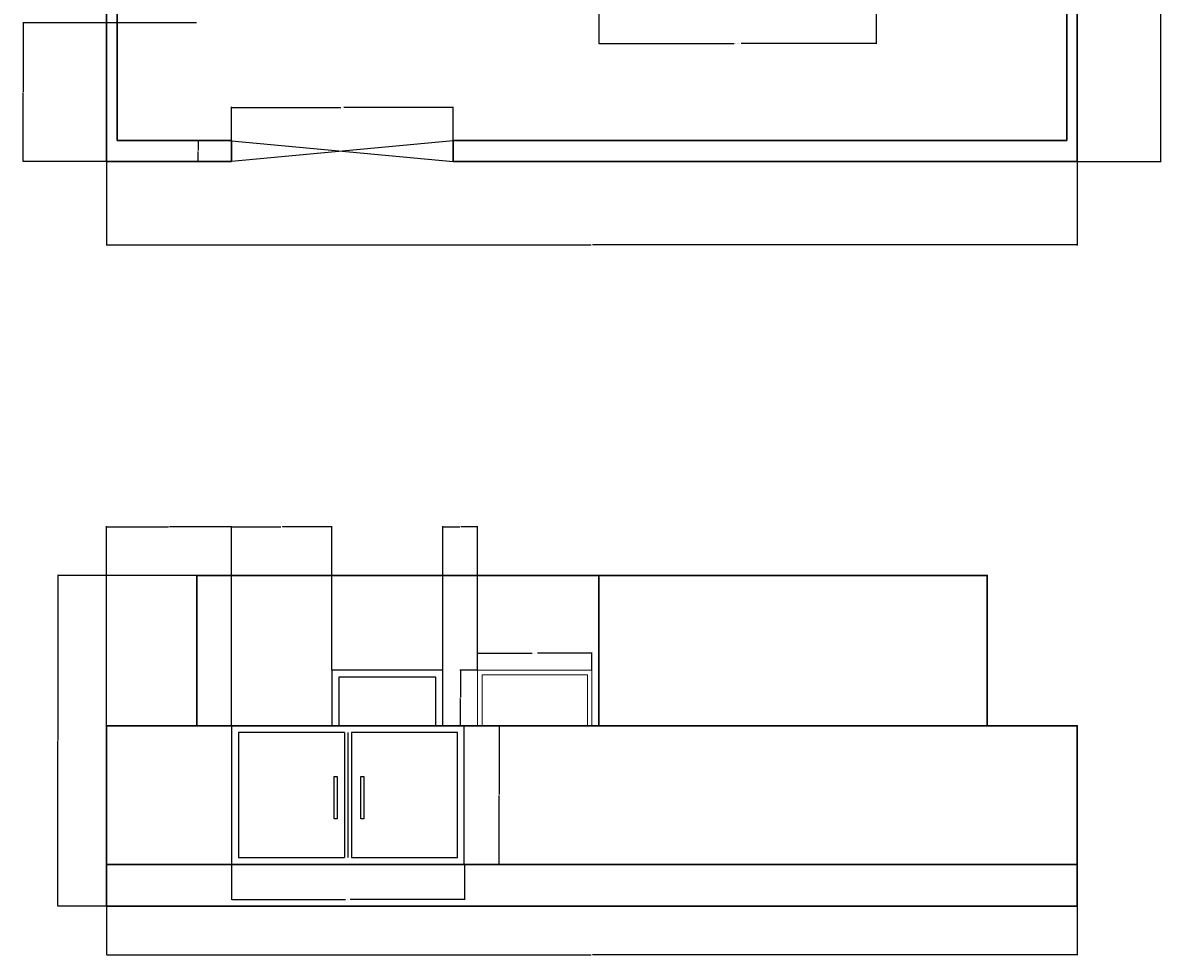
# Model space of a CAD drawing. Units: inches. Extents: x 810 to 2232, y 728 to 1827.
# Tile 1 of 6: x 810 to 1302, y 728 to 1131. Entities that reach past the tile are written whole.
import ezdxf

# ---------------------------------------------------------------- set-up
doc = ezdxf.new("R2010")
doc.units = ezdxf.units.IN
for name, color, linetype, lineweight in [('A-ANNO-DIMS', 2, 'Continuous', 18), ('A-ELEV', 7, 'Continuous', 30), ('A-ELEV-DOOR', 7, 'Continuous', 25), ('A-ELEV-GATE', 7, 'Continuous', 25), ('A-ELEV-GLAZ', 7, 'Continuous', 18), ('A-ELEV-SITE', 7, 'Continuous', 30), ('C-SITE-WALL', 7, 'Continuous', 30), ('GATE', 30, 'Continuous', 25)]:
    doc.layers.add(name, color=color, linetype=linetype, lineweight=lineweight)
doc.styles.get("Standard").update_dxf_attribs({"font": 'arial.ttf'})
doc.dimstyles.get("Standard").update_dxf_attribs({"dimtxt": 0.18, "dimasz": 0.18, "dimexe": 0.18, "dimexo": 0.0625, "dimgap": 0.09, "dimtad": 0, "dimtih": 1, "dimtoh": 1, "dimdec": 4, "dimzin": 0, "dimdsep": 46, "dimtxsty": 'Standard', "dimcen": 0.09, "dimadec": 0, "dimazin": 0, "dimtfac": 1, "dimtdec": 4, "dimtofl": 0, "dimtmove": 0, "dimatfit": 3, "dimfxl": 1, "dimtolj": 1, "dimtzin": 0, "dimarcsym": 0})

# ---------------------------------------------------------------- blocks, each defined once
blk = doc.blocks.new('gate')
at = {"layer": 'GATE'}
for p, q in [((899.83, 1079.94), (995.83, 1070.94)), ((995.83, 1079.94), (899.83, 1070.94))]:
    blk.add_line(p, q, dxfattribs=at)
blk = doc.blocks.new('GATE-DOUBLE-ELEV')
for p, q in [((48.89, 57), (48.89, 3)), ((50.39, 57), (50.39, 3)), ((51.89, 57), (51.89, 3))]:
    blk.add_line(p, q)
for points in [[(0, 0), (100.77, 0), (100.77, 60), (0, 60)], [(44.48, 38.04), (45.81, 38.04), (45.81, 19.7), (44.48, 19.7)], [(55.99, 38.04), (57.32, 38.04), (57.32, 19.7), (55.99, 19.7)]]:
    blk.add_lwpolyline(points, close=True)
for points in [[(48.89, 57), (3, 57), (3, 3), (48.89, 3)], [(51.89, 3), (97.77, 3), (97.77, 57), (51.89, 57)]]:
    blk.add_lwpolyline(points)
blk = doc.blocks.new('DOOR-ENTRY-ELEV-SCREENED')
for points in [[(48, 60), (48, 84), (0, 84), (0, 60)], [(45, 60), (45, 81), (3, 81), (3, 60)], [(0, 0), (48, 0)]]:
    blk.add_lwpolyline(points)
blk = doc.blocks.new('WIN-ELEV-SCREENED')
for points in [[(0, 0), (0, 24), (49.5, 24), (49.5, 0)], [(2, 0), (2, 22), (47.5, 22), (47.5, 0)]]:
    blk.add_lwpolyline(points)
blk = doc.blocks.new('*D37')
at = {"layer": 'A-ANNO-DIMS', "color": 0, "lineweight": -2, "transparency": 16777216}
for p, q in [((899.83, 1080.01), (899.83, 1094.52)), ((900.01, 1094.34), (947.24, 1094.34)), ((995.65, 1094.34), (948.43, 1094.34)), ((995.83, 1080.01), (995.83, 1094.52))]:
    blk.add_line(p, q, dxfattribs=at)
at = {"layer": 'A-ANNO-DIMS', "color": 0, "transparency": 16777216}
for points in [[(900.01, 1094.37), (900.01, 1094.31), (899.83, 1094.34)], [(995.65, 1094.37), (995.65, 1094.31), (995.83, 1094.34)]]:
    blk.add_solid(points, dxfattribs=at)
at = {"layer": 'Defpoints', "color": 0, "transparency": 16777216}
for p in [(995.83, 1094.34), (899.83, 1079.94), (995.83, 1079.94)]:
    blk.add_point(p, dxfattribs=at)
at = {"layer": 'A-ANNO-DIMS', "color": 0, "transparency": 16777216, "insert": (947.83, 1094.34), "char_height": 0.18, "attachment_point": 5}
blk.add_mtext('\\A1;GATE 96', dxfattribs=at)
blk = doc.blocks.new('*D38')
at = {"layer": 'A-ANNO-DIMS', "color": 0, "lineweight": -2, "transparency": 16777216}
for p, q in [((899.77, 1079.94), (885.25, 1079.94)), ((885.43, 1079.76), (885.43, 1075.62)), ((885.43, 1071.12), (885.43, 1075.26)), ((899.77, 1070.94), (885.25, 1070.94))]:
    blk.add_line(p, q, dxfattribs=at)
at = {"layer": 'A-ANNO-DIMS', "color": 0, "transparency": 16777216}
for points in [[(885.4, 1079.76), (885.46, 1079.76), (885.43, 1079.94)], [(885.4, 1071.12), (885.46, 1071.12), (885.43, 1070.94)]]:
    blk.add_solid(points, dxfattribs=at)
at = {"layer": 'Defpoints', "color": 0, "transparency": 16777216}
for p in [(885.43, 1079.94), (899.83, 1079.94), (899.83, 1070.94)]:
    blk.add_point(p, dxfattribs=at)
at = {"layer": 'A-ANNO-DIMS', "color": 0, "transparency": 16777216, "insert": (885.43, 1075.44), "char_height": 0.18, "attachment_point": 5}
blk.add_mtext('\\A1;9', dxfattribs=at)
blk = doc.blocks.new('*D41')
at = {"layer": 'A-ANNO-DIMS', "color": 0, "lineweight": -2, "transparency": 16777216}
for p, q in [((899.83, 766.78), (899.83, 751.54)), ((1000.61, 766.78), (1000.61, 751.54)), ((900.01, 751.72), (949.25, 751.72)), ((1000.43, 751.72), (951.19, 751.72))]:
    blk.add_line(p, q, dxfattribs=at)
at = {"layer": 'A-ANNO-DIMS', "color": 0, "transparency": 16777216}
for points in [[(900.01, 751.75), (900.01, 751.69), (899.83, 751.72)], [(1000.43, 751.75), (1000.43, 751.69), (1000.61, 751.72)]]:
    blk.add_solid(points, dxfattribs=at)
at = {"layer": 'Defpoints', "color": 0, "transparency": 16777216}
for p in [(899.83, 766.84), (1000.61, 766.84), (1000.61, 751.72)]:
    blk.add_point(p, dxfattribs=at)
at = {"layer": 'A-ANNO-DIMS', "color": 0, "transparency": 16777216, "insert": (950.22, 751.72), "char_height": 0.18, "attachment_point": 5}
blk.add_mtext('\\A1;GATE 101 TYP.', dxfattribs=at)
blk = doc.blocks.new('*D42')
at = {"layer": 'A-ANNO-DIMS', "color": 0, "lineweight": -2, "transparency": 16777216}
for p, q in [((1000.67, 826.84), (1015.9, 826.84)), ((1015.72, 826.66), (1015.72, 797.02)), ((1015.72, 767.02), (1015.72, 796.66)), ((1000.67, 766.84), (1015.9, 766.84))]:
    blk.add_line(p, q, dxfattribs=at)
at = {"layer": 'A-ANNO-DIMS', "color": 0, "transparency": 16777216}
for points in [[(1015.69, 826.66), (1015.75, 826.66), (1015.72, 826.84)], [(1015.69, 767.02), (1015.75, 767.02), (1015.72, 766.84)]]:
    blk.add_solid(points, dxfattribs=at)
at = {"layer": 'Defpoints', "color": 0, "transparency": 16777216}
for p in [(1000.61, 826.84), (1015.72, 826.84), (1000.61, 766.84)]:
    blk.add_point(p, dxfattribs=at)
at = {"layer": 'A-ANNO-DIMS', "color": 0, "transparency": 16777216, "insert": (1015.72, 796.84), "char_height": 0.18, "attachment_point": 5}
blk.add_mtext('\\A1;60 TYP.', dxfattribs=at)
blk = doc.blocks.new('*D45')
at = {"layer": 'A-ANNO-DIMS', "color": 0, "lineweight": -2, "transparency": 16777216}
for p, q in [((1006.33, 850.9), (1006.33, 858.45)), ((1006.51, 858.27), (1029.97, 858.27)), ((1055.65, 858.27), (1032.2, 858.27)), ((1055.83, 850.9), (1055.83, 858.45))]:
    blk.add_line(p, q, dxfattribs=at)
at = {"layer": 'A-ANNO-DIMS', "color": 0, "transparency": 16777216}
for points in [[(1006.51, 858.3), (1006.51, 858.24), (1006.33, 858.27)], [(1055.65, 858.3), (1055.65, 858.24), (1055.83, 858.27)]]:
    blk.add_solid(points, dxfattribs=at)
at = {"layer": 'Defpoints', "color": 0, "transparency": 16777216}
for p in [(1055.83, 858.27), (1006.33, 850.84), (1055.83, 850.84)]:
    blk.add_point(p, dxfattribs=at)
at = {"layer": 'A-ANNO-DIMS', "color": 0, "transparency": 16777216, "insert": (1031.08, 858.27), "char_height": 0.18, "attachment_point": 5}
blk.add_mtext('\\A1;WINDOW 50 TYP.', dxfattribs=at)
blk = doc.blocks.new('*D46')
at = {"layer": 'A-ANNO-DIMS', "color": 0, "lineweight": -2, "transparency": 16777216}
for p, q in [((1006.27, 850.84), (998.73, 850.84)), ((998.91, 850.66), (998.91, 839.02)), ((998.91, 827.02), (998.91, 838.66)), ((1006.27, 826.84), (998.73, 826.84))]:
    blk.add_line(p, q, dxfattribs=at)
at = {"layer": 'A-ANNO-DIMS', "color": 0, "transparency": 16777216}
for points in [[(998.88, 850.66), (998.94, 850.66), (998.91, 850.84)], [(998.88, 827.02), (998.94, 827.02), (998.91, 826.84)]]:
    blk.add_solid(points, dxfattribs=at)
at = {"layer": 'Defpoints', "color": 0, "transparency": 16777216}
for p in [(998.91, 850.84), (1006.33, 850.84), (1006.33, 826.84)]:
    blk.add_point(p, dxfattribs=at)
at = {"layer": 'A-ANNO-DIMS', "color": 0, "transparency": 16777216, "insert": (998.91, 838.84), "char_height": 0.18, "attachment_point": 5}
blk.add_mtext('\\A1;24 TYP.', dxfattribs=at)
blk = doc.blocks.new('*D55')
at = {"layer": 'A-ANNO-DIMS', "color": 0, "lineweight": -2, "transparency": 16777216}
for p, q in [((1058.83, 1139.88), (1058.83, 1121.76)), ((1178.83, 1139.88), (1178.83, 1121.76)), ((1059.01, 1121.94), (1117.35, 1121.94)), ((1178.65, 1121.94), (1120.32, 1121.94))]:
    blk.add_line(p, q, dxfattribs=at)
at = {"layer": 'A-ANNO-DIMS', "color": 0, "transparency": 16777216}
for points in [[(1059.01, 1121.97), (1059.01, 1121.91), (1058.83, 1121.94)], [(1178.65, 1121.97), (1178.65, 1121.91), (1178.83, 1121.94)]]:
    blk.add_solid(points, dxfattribs=at)
at = {"layer": 'Defpoints', "color": 0, "transparency": 16777216}
for p in [(1058.83, 1139.94), (1178.83, 1139.94), (1178.83, 1121.94)]:
    blk.add_point(p, dxfattribs=at)
at = {"layer": 'A-ANNO-DIMS', "color": 0, "transparency": 16777216, "insert": (1118.83, 1121.94), "char_height": 0.18, "attachment_point": 5}
blk.add_mtext('\\A1;STAIR FLIGHT 120 TYP.', dxfattribs=at)
blk = doc.blocks.new('*D59')
at = {"layer": 'A-ANNO-DIMS', "color": 0, "lineweight": -2, "transparency": 16777216}
for p, q in [((845.83, 1070.88), (845.83, 1034.66)), ((1265.83, 1070.88), (1265.83, 1034.66)), ((846.01, 1034.84), (1055.54, 1034.84)), ((1265.65, 1034.84), (1056.13, 1034.84))]:
    blk.add_line(p, q, dxfattribs=at)
at = {"layer": 'A-ANNO-DIMS', "color": 0, "transparency": 16777216}
for points in [[(846.01, 1034.87), (846.01, 1034.81), (845.83, 1034.84)], [(1265.65, 1034.87), (1265.65, 1034.81), (1265.83, 1034.84)]]:
    blk.add_solid(points, dxfattribs=at)
at = {"layer": 'Defpoints', "color": 0, "transparency": 16777216}
for p in [(845.83, 1070.94), (1265.83, 1070.94), (1265.83, 1034.84)]:
    blk.add_point(p, dxfattribs=at)
at = {"layer": 'A-ANNO-DIMS', "color": 0, "transparency": 16777216, "insert": (1055.83, 1034.84), "char_height": 0.18, "attachment_point": 5}
blk.add_mtext('\\A1;420', dxfattribs=at)
blk = doc.blocks.new('*D60')
at = {"layer": 'A-ANNO-DIMS', "color": 0, "lineweight": -2, "transparency": 16777216}
for p, q in [((1265.9, 1790.94), (1302.11, 1790.94)), ((1301.93, 1790.76), (1301.93, 1431.12)), ((1301.93, 1071.12), (1301.93, 1430.76)), ((1265.9, 1070.94), (1302.11, 1070.94))]:
    blk.add_line(p, q, dxfattribs=at)
at = {"layer": 'A-ANNO-DIMS', "color": 0, "transparency": 16777216}
for points in [[(1301.9, 1790.76), (1301.96, 1790.76), (1301.93, 1790.94)], [(1301.9, 1071.12), (1301.96, 1071.12), (1301.93, 1070.94)]]:
    blk.add_solid(points, dxfattribs=at)
at = {"layer": 'Defpoints', "color": 0, "transparency": 16777216}
for p in [(1265.83, 1790.94), (1301.93, 1790.94), (1265.83, 1070.94)]:
    blk.add_point(p, dxfattribs=at)
at = {"layer": 'A-ANNO-DIMS', "color": 0, "transparency": 16777216, "insert": (1301.93, 1430.94), "char_height": 0.18, "attachment_point": 5}
blk.add_mtext('\\A1;720', dxfattribs=at)
blk = doc.blocks.new('*D64')
at = {"layer": 'A-ANNO-DIMS', "color": 0, "lineweight": -2, "transparency": 16777216}
for p, q in [((884.77, 1130.94), (809.55, 1130.94)), ((809.73, 1130.76), (809.73, 1101.12)), ((809.73, 1071.12), (809.73, 1100.76)), ((845.77, 1070.94), (809.55, 1070.94))]:
    blk.add_line(p, q, dxfattribs=at)
at = {"layer": 'A-ANNO-DIMS', "color": 0, "transparency": 16777216}
for points in [[(809.7, 1130.76), (809.76, 1130.76), (809.73, 1130.94)], [(809.7, 1071.12), (809.76, 1071.12), (809.73, 1070.94)]]:
    blk.add_solid(points, dxfattribs=at)
at = {"layer": 'Defpoints', "color": 0, "transparency": 16777216}
for p in [(884.83, 1130.94), (809.73, 1070.94), (845.83, 1070.94)]:
    blk.add_point(p, dxfattribs=at)
at = {"layer": 'A-ANNO-DIMS', "color": 0, "transparency": 16777216, "insert": (809.73, 1100.94), "char_height": 0.18, "attachment_point": 5}
blk.add_mtext('\\A1;60', dxfattribs=at)
blk = doc.blocks.new('*D83')
at = {"layer": 'A-ANNO-DIMS', "color": 0, "lineweight": -2, "transparency": 16777216}
for p, q in [((845.83, 748.78), (845.83, 727.56)), ((1265.83, 748.78), (1265.83, 727.56)), ((846.01, 727.74), (1055.54, 727.74)), ((1265.65, 727.74), (1056.13, 727.74))]:
    blk.add_line(p, q, dxfattribs=at)
at = {"layer": 'A-ANNO-DIMS', "color": 0, "transparency": 16777216}
for points in [[(846.01, 727.77), (846.01, 727.71), (845.83, 727.74)], [(1265.65, 727.77), (1265.65, 727.71), (1265.83, 727.74)]]:
    blk.add_solid(points, dxfattribs=at)
at = {"layer": 'Defpoints', "color": 0, "transparency": 16777216}
for p in [(845.83, 748.84), (1265.83, 748.84), (1265.83, 727.74)]:
    blk.add_point(p, dxfattribs=at)
at = {"layer": 'A-ANNO-DIMS', "color": 0, "transparency": 16777216, "insert": (1055.83, 727.74), "char_height": 0.18, "attachment_point": 5}
blk.add_mtext('\\A1;420', dxfattribs=at)
blk = doc.blocks.new('*D84')
at = {"layer": 'A-ANNO-DIMS', "color": 0, "lineweight": -2, "transparency": 16777216}
for p, q in [((884.77, 891.84), (824.55, 891.84)), ((824.73, 891.66), (824.73, 820.52)), ((824.73, 749.02), (824.73, 820.16)), ((845.77, 748.84), (824.55, 748.84))]:
    blk.add_line(p, q, dxfattribs=at)
at = {"layer": 'A-ANNO-DIMS', "color": 0, "transparency": 16777216}
for points in [[(824.7, 891.66), (824.76, 891.66), (824.73, 891.84)], [(824.7, 749.02), (824.76, 749.02), (824.73, 748.84)]]:
    blk.add_solid(points, dxfattribs=at)
at = {"layer": 'Defpoints', "color": 0, "transparency": 16777216}
for p in [(824.73, 891.84), (884.83, 891.84), (845.83, 748.84)]:
    blk.add_point(p, dxfattribs=at)
at = {"layer": 'A-ANNO-DIMS', "color": 0, "transparency": 16777216, "insert": (824.73, 820.34), "char_height": 0.18, "attachment_point": 5}
blk.add_mtext('\\A1;143', dxfattribs=at)
blk = doc.blocks.new('*D85')
at = {"layer": 'A-ANNO-DIMS', "color": 0, "lineweight": -2, "transparency": 16777216}
for p, q in [((845.83, 826.9), (845.83, 913.12)), ((846.01, 912.94), (872.62, 912.94)), ((899.65, 912.94), (873.05, 912.94)), ((899.83, 826.9), (899.83, 913.12))]:
    blk.add_line(p, q, dxfattribs=at)
at = {"layer": 'A-ANNO-DIMS', "color": 0, "transparency": 16777216}
for points in [[(846.01, 912.97), (846.01, 912.91), (845.83, 912.94)], [(899.65, 912.97), (899.65, 912.91), (899.83, 912.94)]]:
    blk.add_solid(points, dxfattribs=at)
at = {"layer": 'Defpoints', "color": 0, "transparency": 16777216}
for p in [(899.83, 912.94), (845.83, 826.84), (899.83, 826.84)]:
    blk.add_point(p, dxfattribs=at)
at = {"layer": 'A-ANNO-DIMS', "color": 0, "transparency": 16777216, "insert": (872.83, 912.94), "char_height": 0.18, "attachment_point": 5}
blk.add_mtext('\\A1;54', dxfattribs=at)
blk = doc.blocks.new('*D86')
at = {"layer": 'A-ANNO-DIMS', "color": 0, "lineweight": -2, "transparency": 16777216}
for p, q in [((899.83, 826.9), (899.83, 913.12)), ((900.01, 912.94), (921.26, 912.94)), ((943.15, 912.94), (921.91, 912.94)), ((943.33, 850.9), (943.33, 913.12))]:
    blk.add_line(p, q, dxfattribs=at)
at = {"layer": 'A-ANNO-DIMS', "color": 0, "transparency": 16777216}
for points in [[(900.01, 912.97), (900.01, 912.91), (899.83, 912.94)], [(943.15, 912.97), (943.15, 912.91), (943.33, 912.94)]]:
    blk.add_solid(points, dxfattribs=at)
at = {"layer": 'Defpoints', "color": 0, "transparency": 16777216}
for p in [(943.33, 912.94), (943.33, 850.84), (899.83, 826.84)]:
    blk.add_point(p, dxfattribs=at)
at = {"layer": 'A-ANNO-DIMS', "color": 0, "transparency": 16777216, "insert": (921.58, 912.94), "char_height": 0.18, "attachment_point": 5}
blk.add_mtext('\\A1;43.5', dxfattribs=at)
blk = doc.blocks.new('*D87')
at = {"layer": 'A-ANNO-DIMS', "color": 0, "lineweight": -2, "transparency": 16777216}
for p, q in [((991.33, 850.9), (991.33, 913.12)), ((991.51, 912.94), (998.62, 912.94)), ((1006.15, 912.94), (999.05, 912.94)), ((1006.33, 850.9), (1006.33, 913.12))]:
    blk.add_line(p, q, dxfattribs=at)
at = {"layer": 'A-ANNO-DIMS', "color": 0, "transparency": 16777216}
for points in [[(991.51, 912.97), (991.51, 912.91), (991.33, 912.94)], [(1006.15, 912.97), (1006.15, 912.91), (1006.33, 912.94)]]:
    blk.add_solid(points, dxfattribs=at)
at = {"layer": 'Defpoints', "color": 0, "transparency": 16777216}
for p in [(1006.33, 912.94), (991.33, 850.84), (1006.33, 850.84)]:
    blk.add_point(p, dxfattribs=at)
at = {"layer": 'A-ANNO-DIMS', "color": 0, "transparency": 16777216, "insert": (998.83, 912.94), "char_height": 0.18, "attachment_point": 5}
blk.add_mtext('\\A1;15', dxfattribs=at)

msp = doc.modelspace()

# ---------------------------------------------------------------- linework, layer by layer
at = {"layer": 'A-ELEV'}
for points in [[(1058.8341, 826.8406), (1058.8341, 891.8406), (884.8341, 891.8406), (884.8341, 826.8406)], [(1058.8341, 826.8406), (1058.8341, 891.8406), (1226.8341, 891.8406), (1226.8341, 826.8406)], [(884.8341, 766.8406), (1058.8341, 766.8406)], [(1226.8341, 766.8406), (1058.8341, 766.8406)]]:
    msp.add_lwpolyline(points, dxfattribs=at)
at = {"layer": 'A-ELEV-SITE'}
for points in [[(845.8341, 766.8406), (1265.8341, 766.8406), (1265.8341, 826.8406), (845.8341, 826.8406)], [(845.8341, 766.8406), (1265.8341, 766.8406), (1265.8341, 748.8406), (845.8341, 748.8406)]]:
    msp.add_lwpolyline(points, close=True, dxfattribs=at)
at = {"layer": 'C-SITE-WALL'}
for p, q in [((845.8341, 1070.9426), (845.8341, 1790.9426)), ((1265.8341, 1790.9426), (1265.8341, 1070.9426)), ((850.3341, 1079.9426), (850.3341, 1786.4426)), ((1261.3341, 1786.4426), (1261.3341, 1079.9426)), ((899.8341, 1079.9426), (850.3341, 1079.9426)), ((899.8341, 1079.9426), (899.8341, 1070.9426)), ((1261.3341, 1079.9426), (995.8341, 1079.9426)), ((995.8341, 1079.9426), (995.8341, 1070.9426)), ((899.8341, 1070.9426), (845.8341, 1070.9426)), ((1265.8341, 1070.9426), (995.8341, 1070.9426))]:
    msp.add_line(p, q, dxfattribs=at)

# ---------------------------------------------------------------- block references
at = {"layer": 'A-ELEV-DOOR'}
msp.add_blockref('DOOR-ENTRY-ELEV-SCREENED', (943.334, 766.841), dxfattribs=at)
at = {"layer": 'A-ELEV-GATE'}
msp.add_blockref('GATE-DOUBLE-ELEV', (899.834, 766.841), dxfattribs=at)
at = {"layer": 'A-ELEV-GLAZ'}
msp.add_blockref('WIN-ELEV-SCREENED', (1006.334, 826.841), dxfattribs=at)
at = {"layer": 'GATE'}
msp.add_blockref('gate', (0, 0), dxfattribs=at)

# ---------------------------------------------------------------- dimensions: what is measured, and where the dimension line sits
at = {"layer": 'A-ANNO-DIMS'}
for base, p1, p2, picture, middle in [((1301.9341, 1790.9426), (1265.8341, 1070.9426), (1265.8341, 1790.9426), '*D60', (1301.9341, 1430.9426)), ((809.7341, 1070.9426), (884.8341, 1130.9426), (845.8341, 1070.9426), '*D64', (809.7341, 1100.9426)), ((885.4341, 1079.9426), (899.8341, 1070.9426), (899.8341, 1079.9426), '*D38', (885.4341, 1075.4426)), ((824.7341, 891.8406), (845.8341, 748.8406), (884.8341, 891.8406), '*D84', (824.7341, 820.3406))]:
    dim = msp.add_linear_dim(base=base, p1=p1, p2=p2, angle=90, dimstyle='Standard', override={"dimdec": 0, "dimlfac": 1, "dimrnd": 0, "dimzin": 0, "dimdsep": 46, "dimlunit": 2}, dxfattribs=at)
    dim.commit()
    dim.dimension.update_dxf_attribs({"geometry": picture, "text_midpoint": middle})
for base, p1, p2, text, picture, middle in [((1178.8341, 1121.9426), (1058.8341, 1139.9426), (1178.8341, 1139.9426), 'STAIR FLIGHT <> TYP.', '*D55', (1118.8341, 1121.9426)), ((995.8341, 1094.3426), (899.8341, 1079.9426), (995.8341, 1079.9426), 'GATE <>', '*D37', (947.8341, 1094.3426)), ((1055.8340622384, 858.265615579), (1006.3340622384, 850.840615579), (1055.8340622384, 850.840615579), 'WINDOW <> TYP.', '*D45', (1031.0840622384, 858.265615579)), ((1000.6051, 751.725), (899.8341, 766.8406), (1000.6051, 766.8406), 'GATE <> TYP.', '*D41', (950.2196, 751.725))]:
    dim = msp.add_linear_dim(base=base, p1=p1, p2=p2, text=text, dimstyle='Standard', override={"dimdec": 0, "dimlfac": 1, "dimrnd": 0, "dimzin": 0, "dimdsep": 46, "dimlunit": 2}, dxfattribs=at)
    dim.commit()
    dim.dimension.update_dxf_attribs({"geometry": picture, "text_midpoint": middle})
for base, p1, p2, override, picture, middle in [((1265.8341, 1034.8426), (845.8341, 1070.9426), (1265.8341, 1070.9426), {"dimdec": 0, "dimlfac": 1, "dimrnd": 0, "dimzin": 0, "dimdsep": 46, "dimlunit": 2}, '*D59', (1055.8341, 1034.8426)), ((899.8341, 912.9406), (845.8341, 826.8406), (899.8341, 826.8406), {"dimdec": 0, "dimlfac": 1, "dimrnd": 0, "dimzin": 0, "dimdsep": 46, "dimlunit": 2}, '*D85', (872.8341, 912.9406)), ((943.3341, 912.9406), (899.8341, 826.8406), (943.3341, 850.8406), {"dimdec": 1, "dimlfac": 1, "dimrnd": 0, "dimzin": 0, "dimdsep": 46, "dimlunit": 2}, '*D86', (921.5841, 912.9406)), ((1006.3341, 912.9406), (991.3341, 850.8406), (1006.3341, 850.8406), {"dimdec": 0, "dimlfac": 1, "dimrnd": 0, "dimzin": 0, "dimdsep": 46, "dimlunit": 2}, '*D87', (998.8341, 912.9406)), ((1265.8341, 727.7406), (845.8341, 748.8406), (1265.8341, 748.8406), {"dimdec": 0, "dimlfac": 1, "dimrnd": 0, "dimzin": 0, "dimdsep": 46, "dimlunit": 2}, '*D83', (1055.8341, 727.7406))]:
    dim = msp.add_linear_dim(base=base, p1=p1, p2=p2, dimstyle='Standard', override=override, dxfattribs=at)
    dim.commit()
    dim.dimension.update_dxf_attribs({"geometry": picture, "text_midpoint": middle})
for base, p1, p2, picture, middle in [((998.9091, 850.8406), (1006.3341, 826.8406), (1006.3341, 850.8406), '*D46', (998.9091, 838.8406)), ((1015.7208, 826.8406), (1000.6051, 766.8406), (1000.6051, 826.8406), '*D42', (1015.7208, 796.8406))]:
    dim = msp.add_linear_dim(base=base, p1=p1, p2=p2, angle=90, text='<> TYP.', dimstyle='Standard', override={"dimdec": 0, "dimlfac": 1, "dimrnd": 0, "dimzin": 0, "dimdsep": 46, "dimlunit": 2}, dxfattribs=at)
    dim.commit()
    dim.dimension.update_dxf_attribs({"geometry": picture, "text_midpoint": middle})

doc.saveas('drawing.dxf')
